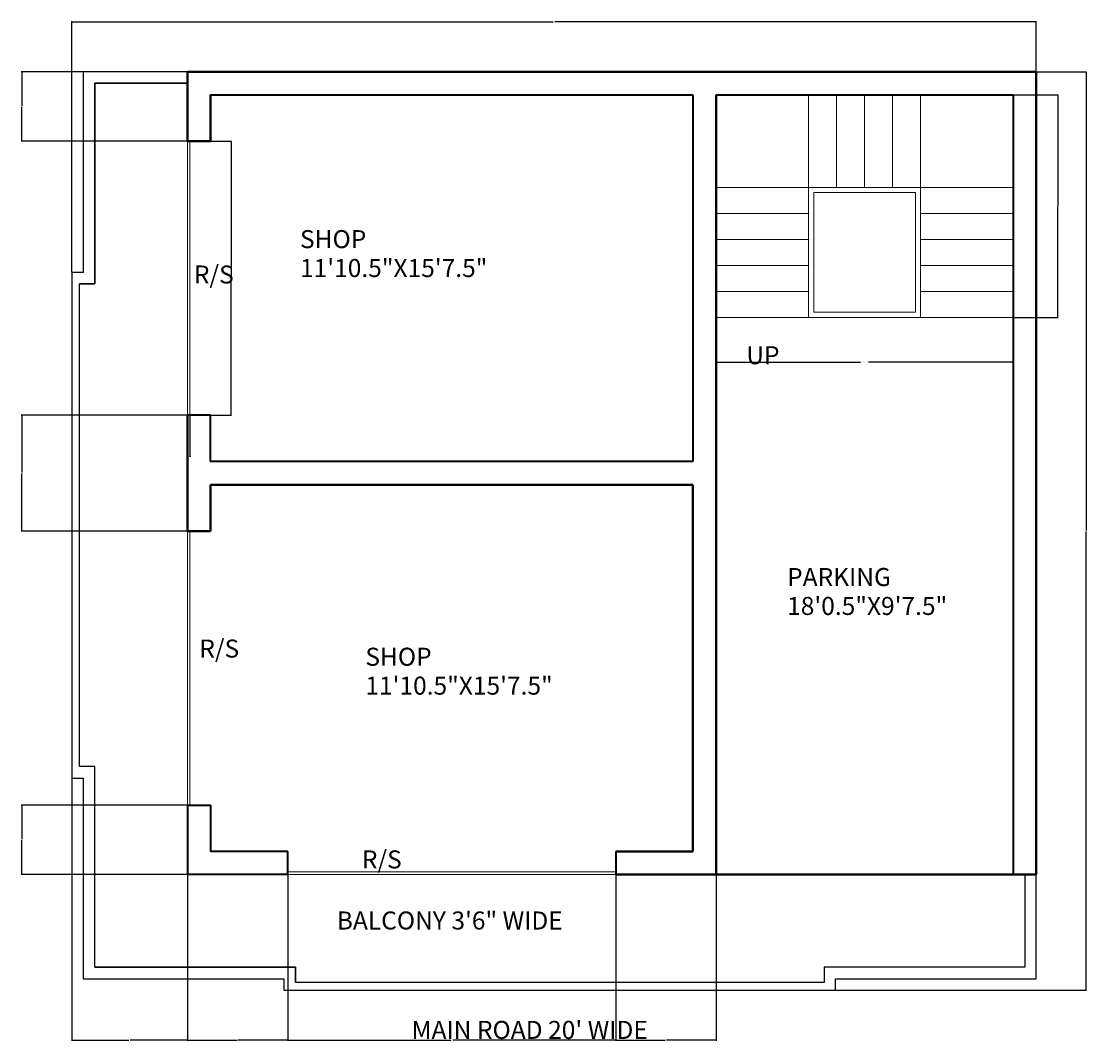
# Model space of a CAD drawing. Units: millimetres. Extents: x 2284 to 2706, y 1197 to 2041.
# Tile 3 of 3: x 2284 to 2698, y 1645 to 2041. Entities that reach past the tile are written whole.
import ezdxf

# ---------------------------------------------------------------- set-up
doc = ezdxf.new("R2010")
doc.units = ezdxf.units.MM
for name, color, linetype, lineweight in [('A-ANNO-DIMS', 2, 'Continuous', 18), ('A-ANNO-TEXT', 7, 'Continuous', 30), ('A-AREA-IDEN', 7, 'Continuous', 30), ('A-CONS', 67, 'Continuous', 13), ('A-DOOR', 7, 'Continuous', 18)]:
    doc.layers.add(name, color=color, linetype=linetype, lineweight=lineweight)
for name, color, linetype, lineweight, true_color in [('A-FLOR-STRS', 67, 'Continuous', 18, 0x727430), ('A-WALL', 11, 'Continuous', 35, 0xf27172), ('A-WALL-PRPT', 143, 'Continuous', 25, 0x7aafdf)]:
    doc.layers.add(name, color=color, linetype=linetype, lineweight=lineweight, true_color=true_color)
doc.styles.get("Standard").update_dxf_attribs({"font": 'arial.ttf'})
doc.dimstyles.get("Standard").update_dxf_attribs({"dimtxt": 0.18, "dimasz": 0.18, "dimexe": 0.18, "dimexo": 0.0625, "dimgap": 0.09, "dimtad": 0, "dimtih": 1, "dimtoh": 1, "dimdec": 4, "dimzin": 0, "dimdsep": 46, "dimtxsty": 'Standard', "dimcen": 0.09, "dimadec": 0, "dimazin": 0, "dimtfac": 1, "dimtdec": 4, "dimtofl": 0, "dimtmove": 0, "dimatfit": 3, "dimfxl": 1, "dimtolj": 1, "dimtzin": 0, "dimarcsym": 0})

# ---------------------------------------------------------------- blocks, each defined once
blk = doc.blocks.new('STAIR-U-RETURN')
for p, q in [((0, 86.5), (36, 86.5)), ((36, 86.5), (36, 50.5)), ((46.87, 50.5), (46.87, 86.5)), ((46.87, 86.5), (46.87, 50.5)), ((57.75, 50.5), (57.75, 86.5)), ((57.75, 86.5), (57.75, 50.5)), ((68.62, 50.5), (68.62, 86.5)), ((79.5, 50.5), (79.5, 86.5)), ((115.5, 50.5), (0, 50.5)), ((36, 50.5), (36, 0)), ((36, 50.5), (79.5, 50.5)), ((79.5, 0), (79.5, 50.5)), ((38, 48.5), (38, 2)), ((77.5, 48.5), (38, 48.5)), ((77.5, 2), (77.5, 48.5)), ((36, 40.4), (0, 40.4)), ((0, 40.4), (36, 40.4)), ((36, 40.4), (36, 30.3)), ((79.5, 40.4), (79.5, 30.3)), ((79.5, 40.4), (115.5, 40.4)), ((115.5, 40.4), (79.5, 40.4)), ((36, 30.3), (0, 30.3)), ((0, 30.3), (36, 30.3)), ((36, 30.3), (36, 20.2)), ((79.5, 30.3), (79.5, 20.2)), ((79.5, 30.3), (115.5, 30.3)), ((115.5, 30.3), (79.5, 30.3)), ((36, 20.2), (0, 20.2)), ((0, 20.2), (36, 20.2)), ((36, 20.2), (36, 10.1)), ((79.5, 20.2), (79.5, 10.1)), ((79.5, 20.2), (115.5, 20.2)), ((115.5, 20.2), (79.5, 20.2)), ((36, 10.1), (0, 10.1)), ((79.5, 10.1), (115.5, 10.1)), ((0, 0), (115.5, 0)), ((38, 2), (77.5, 2))]:
    blk.add_line(p, q)
blk = doc.blocks.new('DOOR-ROLL-SIDE')
for p, q in [((0, 106.5), (0, 0)), ((1, 106.5), (1, 0))]:
    blk.add_line(p, q)
blk = doc.blocks.new('*D7')
at = {"layer": 'A-ANNO-DIMS', "color": 0, "lineweight": -2, "transparency": 16777216}
for p, q in [((2554.18, 1925.73), (2554.18, 1908.29)), ((2669.68, 1925.73), (2669.68, 1908.29)), ((2554.36, 1908.47), (2610.37, 1908.47)), ((2669.5, 1908.47), (2613.49, 1908.47))]:
    blk.add_line(p, q, dxfattribs=at)
at = {"layer": 'A-ANNO-DIMS', "color": 0, "transparency": 16777216}
for points in [[(2554.36, 1908.5), (2554.36, 1908.44), (2554.18, 1908.47)], [(2669.5, 1908.5), (2669.5, 1908.44), (2669.68, 1908.47)]]:
    blk.add_solid(points, dxfattribs=at)
at = {"layer": 'Defpoints', "color": 0, "transparency": 16777216}
for p in [(2554.18, 1925.79), (2669.68, 1925.79), (2669.68, 1908.47)]:
    blk.add_point(p, dxfattribs=at)
at = {"layer": 'A-ANNO-DIMS', "color": 0, "transparency": 16777216, "insert": (2611.93, 1908.47), "char_height": 0.18, "attachment_point": 5}
blk.add_mtext('\\A1;RETURN STAIR 116 TYP.', dxfattribs=at)
blk = doc.blocks.new('*D8')
at = {"layer": 'A-ANNO-DIMS', "color": 0, "lineweight": -2, "transparency": 16777216}
for p, q in [((2669.74, 2012.29), (2687.19, 2012.29)), ((2687.01, 2012.11), (2687.01, 1969.22)), ((2687.01, 1925.97), (2687.01, 1968.86)), ((2669.74, 1925.79), (2687.19, 1925.79))]:
    blk.add_line(p, q, dxfattribs=at)
at = {"layer": 'A-ANNO-DIMS', "color": 0, "transparency": 16777216}
for points in [[(2686.98, 2012.11), (2687.04, 2012.11), (2687.01, 2012.29)], [(2686.98, 1925.97), (2687.04, 1925.97), (2687.01, 1925.79)]]:
    blk.add_solid(points, dxfattribs=at)
at = {"layer": 'Defpoints', "color": 0, "transparency": 16777216}
for p in [(2669.68, 2012.29), (2687.01, 2012.29), (2669.68, 1925.79)]:
    blk.add_point(p, dxfattribs=at)
at = {"layer": 'A-ANNO-DIMS', "color": 0, "transparency": 16777216, "insert": (2687.01, 1969.04), "char_height": 0.18, "attachment_point": 5}
blk.add_mtext('\\A1;87 TYP.', dxfattribs=at)
blk = doc.blocks.new('*D9')
at = {"layer": 'A-ANNO-DIMS', "color": 0, "lineweight": -2, "transparency": 16777216}
for p, q in [((2349.74, 1994.29), (2365.84, 1994.29)), ((2365.66, 1994.11), (2365.66, 1941.23)), ((2365.66, 1887.97), (2365.66, 1940.86)), ((2349.74, 1887.79), (2365.84, 1887.79))]:
    blk.add_line(p, q, dxfattribs=at)
at = {"layer": 'A-ANNO-DIMS', "color": 0, "transparency": 16777216}
for points in [[(2365.63, 1994.11), (2365.69, 1994.11), (2365.66, 1994.29)], [(2365.63, 1887.97), (2365.69, 1887.97), (2365.66, 1887.79)]]:
    blk.add_solid(points, dxfattribs=at)
at = {"layer": 'Defpoints', "color": 0, "transparency": 16777216}
for p in [(2349.68, 1994.29), (2365.66, 1994.29), (2349.68, 1887.79)]:
    blk.add_point(p, dxfattribs=at)
at = {"layer": 'A-ANNO-DIMS', "color": 0, "transparency": 16777216, "insert": (2365.66, 1941.04), "char_height": 0.18, "attachment_point": 5}
blk.add_mtext('\\A1;SHUTTER 107 TYP.', dxfattribs=at)
blk = doc.blocks.new('*D10')
at = {"layer": 'A-ANNO-DIMS', "color": 0, "lineweight": -2, "transparency": 16777216}
for p, q in [((2348.68, 1887.73), (2348.68, 1871.64)), ((2349.68, 1887.73), (2349.68, 1871.64)), ((2348.5, 1871.82), (2348.32, 1871.82)), ((2349.86, 1871.82), (2350.04, 1871.82))]:
    blk.add_line(p, q, dxfattribs=at)
at = {"layer": 'A-ANNO-DIMS', "color": 0, "transparency": 16777216}
for points in [[(2348.5, 1871.85), (2348.5, 1871.79), (2348.68, 1871.82)], [(2349.86, 1871.85), (2349.86, 1871.79), (2349.68, 1871.82)]]:
    blk.add_solid(points, dxfattribs=at)
at = {"layer": 'Defpoints', "color": 0, "transparency": 16777216}
for p in [(2348.68, 1887.79), (2349.68, 1887.79), (2349.68, 1871.82)]:
    blk.add_point(p, dxfattribs=at)
at = {"layer": 'A-ANNO-DIMS', "color": 0, "transparency": 16777216, "insert": (2349.18, 1871.82), "char_height": 0.18, "attachment_point": 5}
blk.add_mtext('\\A1;1 TYP.', dxfattribs=at)
blk = doc.blocks.new('*D19')
at = {"layer": 'A-ANNO-DIMS', "color": 0, "lineweight": -2, "transparency": 16777216}
for p, q in [((2303.68, 1943.35), (2303.68, 2040.87)), ((2303.86, 2040.69), (2490.89, 2040.69)), ((2678.5, 2040.69), (2491.47, 2040.69)), ((2678.68, 2021.35), (2678.68, 2040.87))]:
    blk.add_line(p, q, dxfattribs=at)
at = {"layer": 'A-ANNO-DIMS', "color": 0, "transparency": 16777216}
for points in [[(2303.86, 2040.72), (2303.86, 2040.66), (2303.68, 2040.69)], [(2678.5, 2040.72), (2678.5, 2040.66), (2678.68, 2040.69)]]:
    blk.add_solid(points, dxfattribs=at)
at = {"layer": 'Defpoints', "color": 0, "transparency": 16777216}
for p in [(2678.68, 2040.69), (2678.68, 2021.29), (2303.68, 1943.29)]:
    blk.add_point(p, dxfattribs=at)
at = {"layer": 'A-ANNO-DIMS', "color": 0, "transparency": 16777216, "insert": (2491.18, 2040.69), "char_height": 0.18, "attachment_point": 5}
blk.add_mtext('\\A1;375', dxfattribs=at)
blk = doc.blocks.new('*D20')
at = {"layer": 'A-ANNO-DIMS', "color": 0, "lineweight": -2, "transparency": 16777216}
for p, q in [((2678.74, 2021.29), (2698.26, 2021.29)), ((2698.08, 2021.11), (2698.08, 1842.97)), ((2698.08, 1664.47), (2698.08, 1842.61)), ((2600.74, 1664.29), (2698.26, 1664.29))]:
    blk.add_line(p, q, dxfattribs=at)
at = {"layer": 'A-ANNO-DIMS', "color": 0, "transparency": 16777216}
for points in [[(2698.05, 2021.11), (2698.11, 2021.11), (2698.08, 2021.29)], [(2698.05, 1664.47), (2698.11, 1664.47), (2698.08, 1664.29)]]:
    blk.add_solid(points, dxfattribs=at)
at = {"layer": 'Defpoints', "color": 0, "transparency": 16777216}
for p in [(2678.68, 2021.29), (2698.08, 2021.29), (2600.68, 1664.29)]:
    blk.add_point(p, dxfattribs=at)
at = {"layer": 'A-ANNO-DIMS', "color": 0, "transparency": 16777216, "insert": (2698.08, 1842.79), "char_height": 0.18, "attachment_point": 5}
blk.add_mtext('\\A1;357', dxfattribs=at)
blk = doc.blocks.new('*D21')
at = {"layer": 'A-ANNO-DIMS', "color": 0, "lineweight": -2, "transparency": 16777216}
for p, q in [((2348.62, 2021.29), (2284.1, 2021.29)), ((2284.28, 2021.11), (2284.28, 2007.97)), ((2284.28, 1994.47), (2284.28, 2007.61)), ((2348.62, 1994.29), (2284.1, 1994.29))]:
    blk.add_line(p, q, dxfattribs=at)
at = {"layer": 'A-ANNO-DIMS', "color": 0, "transparency": 16777216}
for points in [[(2284.25, 2021.11), (2284.31, 2021.11), (2284.28, 2021.29)], [(2284.25, 1994.47), (2284.31, 1994.47), (2284.28, 1994.29)]]:
    blk.add_solid(points, dxfattribs=at)
at = {"layer": 'Defpoints', "color": 0, "transparency": 16777216}
for p in [(2284.28, 2021.29), (2348.68, 2021.29), (2348.68, 1994.29)]:
    blk.add_point(p, dxfattribs=at)
at = {"layer": 'A-ANNO-DIMS', "color": 0, "transparency": 16777216, "insert": (2284.28, 2007.79), "char_height": 0.18, "attachment_point": 5}
blk.add_mtext('\\A1;27', dxfattribs=at)
blk = doc.blocks.new('*D22')
at = {"layer": 'A-ANNO-DIMS', "color": 0, "lineweight": -2, "transparency": 16777216}
for p, q in [((2348.62, 1887.79), (2284.1, 1887.79)), ((2284.28, 1887.61), (2284.28, 1865.47)), ((2284.28, 1842.97), (2284.28, 1865.11)), ((2348.62, 1842.79), (2284.1, 1842.79))]:
    blk.add_line(p, q, dxfattribs=at)
at = {"layer": 'A-ANNO-DIMS', "color": 0, "transparency": 16777216}
for points in [[(2284.25, 1887.61), (2284.31, 1887.61), (2284.28, 1887.79)], [(2284.25, 1842.97), (2284.31, 1842.97), (2284.28, 1842.79)]]:
    blk.add_solid(points, dxfattribs=at)
at = {"layer": 'Defpoints', "color": 0, "transparency": 16777216}
for p in [(2284.28, 1887.79), (2348.68, 1887.79), (2348.68, 1842.79)]:
    blk.add_point(p, dxfattribs=at)
at = {"layer": 'A-ANNO-DIMS', "color": 0, "transparency": 16777216, "insert": (2284.28, 1865.29), "char_height": 0.18, "attachment_point": 5}
blk.add_mtext('\\A1;45', dxfattribs=at)
blk = doc.blocks.new('*D23')
at = {"layer": 'A-ANNO-DIMS', "color": 0, "lineweight": -2, "transparency": 16777216}
for p, q in [((2348.62, 1736.29), (2284.1, 1736.29)), ((2284.28, 1736.11), (2284.28, 1722.97)), ((2284.28, 1709.47), (2284.28, 1722.61)), ((2348.62, 1709.29), (2284.1, 1709.29))]:
    blk.add_line(p, q, dxfattribs=at)
at = {"layer": 'A-ANNO-DIMS', "color": 0, "transparency": 16777216}
for points in [[(2284.25, 1736.11), (2284.31, 1736.11), (2284.28, 1736.29)], [(2284.25, 1709.47), (2284.31, 1709.47), (2284.28, 1709.29)]]:
    blk.add_solid(points, dxfattribs=at)
at = {"layer": 'Defpoints', "color": 0, "transparency": 16777216}
for p in [(2284.28, 1736.29), (2348.68, 1736.29), (2348.68, 1709.29)]:
    blk.add_point(p, dxfattribs=at)
at = {"layer": 'A-ANNO-DIMS', "color": 0, "transparency": 16777216, "insert": (2284.28, 1722.79), "char_height": 0.18, "attachment_point": 5}
blk.add_mtext('\\A1;27', dxfattribs=at)
blk = doc.blocks.new('*D24')
at = {"layer": 'A-ANNO-DIMS', "color": 0, "lineweight": -2, "transparency": 16777216}
for p, q in [((2303.68, 1746.73), (2303.68, 1644.71)), ((2348.68, 1709.23), (2348.68, 1644.71)), ((2303.86, 1644.89), (2325.96, 1644.89)), ((2348.5, 1644.89), (2326.4, 1644.89))]:
    blk.add_line(p, q, dxfattribs=at)
at = {"layer": 'A-ANNO-DIMS', "color": 0, "transparency": 16777216}
for points in [[(2303.86, 1644.92), (2303.86, 1644.86), (2303.68, 1644.89)], [(2348.5, 1644.92), (2348.5, 1644.86), (2348.68, 1644.89)]]:
    blk.add_solid(points, dxfattribs=at)
at = {"layer": 'Defpoints', "color": 0, "transparency": 16777216}
for p in [(2303.68, 1746.79), (2348.68, 1709.29), (2348.68, 1644.89)]:
    blk.add_point(p, dxfattribs=at)
at = {"layer": 'A-ANNO-DIMS', "color": 0, "transparency": 16777216, "insert": (2326.18, 1644.89), "char_height": 0.18, "attachment_point": 5}
blk.add_mtext('\\A1;45', dxfattribs=at)
blk = doc.blocks.new('*D25')
at = {"layer": 'A-ANNO-DIMS', "color": 0, "lineweight": -2, "transparency": 16777216}
for p, q in [((2348.68, 1709.23), (2348.68, 1644.71)), ((2387.68, 1709.23), (2387.68, 1644.71)), ((2348.86, 1644.89), (2367.96, 1644.89)), ((2387.5, 1644.89), (2368.4, 1644.89))]:
    blk.add_line(p, q, dxfattribs=at)
at = {"layer": 'A-ANNO-DIMS', "color": 0, "transparency": 16777216}
for points in [[(2348.86, 1644.92), (2348.86, 1644.86), (2348.68, 1644.89)], [(2387.5, 1644.92), (2387.5, 1644.86), (2387.68, 1644.89)]]:
    blk.add_solid(points, dxfattribs=at)
at = {"layer": 'Defpoints', "color": 0, "transparency": 16777216}
for p in [(2348.68, 1709.29), (2387.68, 1709.29), (2387.68, 1644.89)]:
    blk.add_point(p, dxfattribs=at)
at = {"layer": 'A-ANNO-DIMS', "color": 0, "transparency": 16777216, "insert": (2368.18, 1644.89), "char_height": 0.18, "attachment_point": 5}
blk.add_mtext('\\A1;39', dxfattribs=at)
blk = doc.blocks.new('*D26')
at = {"layer": 'A-ANNO-DIMS', "color": 0, "lineweight": -2, "transparency": 16777216}
for p, q in [((2387.68, 1709.23), (2387.68, 1644.71)), ((2515.18, 1709.23), (2515.18, 1644.71)), ((2387.86, 1644.89), (2451.04, 1644.89)), ((2515, 1644.89), (2451.82, 1644.89))]:
    blk.add_line(p, q, dxfattribs=at)
at = {"layer": 'A-ANNO-DIMS', "color": 0, "transparency": 16777216}
for points in [[(2387.86, 1644.92), (2387.86, 1644.86), (2387.68, 1644.89)], [(2515, 1644.92), (2515, 1644.86), (2515.18, 1644.89)]]:
    blk.add_solid(points, dxfattribs=at)
at = {"layer": 'Defpoints', "color": 0, "transparency": 16777216}
for p in [(2387.68, 1709.29), (2515.18, 1709.29), (2515.18, 1644.89)]:
    blk.add_point(p, dxfattribs=at)
at = {"layer": 'A-ANNO-DIMS', "color": 0, "transparency": 16777216, "insert": (2451.43, 1644.89), "char_height": 0.18, "attachment_point": 5}
blk.add_mtext('\\A1;127.5', dxfattribs=at)
blk = doc.blocks.new('*D27')
at = {"layer": 'A-ANNO-DIMS', "color": 0, "lineweight": -2, "transparency": 16777216}
for p, q in [((2515.18, 1709.23), (2515.18, 1644.71)), ((2554.18, 1709.23), (2554.18, 1644.71)), ((2515.36, 1644.89), (2534.46, 1644.89)), ((2554, 1644.89), (2534.9, 1644.89))]:
    blk.add_line(p, q, dxfattribs=at)
at = {"layer": 'A-ANNO-DIMS', "color": 0, "transparency": 16777216}
for points in [[(2515.36, 1644.92), (2515.36, 1644.86), (2515.18, 1644.89)], [(2554, 1644.92), (2554, 1644.86), (2554.18, 1644.89)]]:
    blk.add_solid(points, dxfattribs=at)
at = {"layer": 'Defpoints', "color": 0, "transparency": 16777216}
for p in [(2515.18, 1709.29), (2554.18, 1709.29), (2554.18, 1644.89)]:
    blk.add_point(p, dxfattribs=at)
at = {"layer": 'A-ANNO-DIMS', "color": 0, "transparency": 16777216, "insert": (2534.68, 1644.89), "char_height": 0.18, "attachment_point": 5}
blk.add_mtext('\\A1;39', dxfattribs=at)

msp = doc.modelspace()

# ---------------------------------------------------------------- linework, layer by layer
at = {"layer": 'A-CONS'}
for p in [(2601.06, 1976.29), (2611.93, 1976.29), (2622.81, 1976.29), (2590.18, 1966.19), (2633.68, 1966.19), (2590.18, 1956.09), (2633.68, 1956.09), (2590.18, 1945.99), (2633.68, 1945.99), (2590.18, 1935.89), (2633.68, 1935.89)]:
    msp.add_point(p, dxfattribs=at)
at = {"layer": 'A-DOOR'}
for p, q in [((2349.68, 1736.29), (2348.68, 1736.29)), ((2349.68, 1736.29), (2348.68, 1736.29)), ((2349.68, 1736.29), (2348.68, 1736.29)), ((2387.68, 1710.29), (2387.68, 1709.29)), ((2387.68, 1710.29), (2515.18, 1710.29)), ((2387.68, 1709.29), (2515.18, 1709.29))]:
    msp.add_line(p, q, dxfattribs=at)
at = {"layer": 'A-FLOR-STRS'}
for p, q in [((2554.18, 2012.29), (2584.18, 2012.29)), ((2554.18, 2012.29), (2554.18, 1982.29)), ((2590.18, 2012.29), (2590.18, 1976.29)), ((2669.68, 2012.29), (2633.68, 2012.29)), ((2633.68, 2012.29), (2633.68, 1976.29)), ((2669.68, 2012.29), (2639.68, 2012.29)), ((2601.06, 1976.29), (2611.93, 1976.29)), ((2611.93, 1976.29), (2622.81, 1976.29)), ((2631.68, 1976.29), (2669.68, 1976.29)), ((2633.68, 1976.29), (2633.68, 1925.79)), ((2592.18, 1927.79), (2592.18, 1974.29)), ((2592.18, 1974.29), (2631.68, 1974.29)), ((2631.68, 1974.29), (2631.68, 1927.79)), ((2592.18, 1927.79), (2631.68, 1927.79)), ((2590.18, 1925.79), (2554.18, 1925.79)), ((2590.18, 1925.79), (2633.68, 1925.79)), ((2590.18, 1925.79), (2633.68, 1925.79)), ((2669.68, 1925.79), (2633.68, 1925.79))]:
    msp.add_line(p, q, dxfattribs=at)
at = {"layer": 'A-WALL'}
for p, q in [((2348.68, 2021.29), (2678.68, 2021.29)), ((2348.68, 2021.29), (2357.68, 2021.29)), ((2348.68, 1994.29), (2348.68, 2021.29)), ((2678.68, 2021.29), (2348.68, 2021.29)), ((2348.68, 2021.29), (2348.68, 1994.29)), ((2678.68, 2021.29), (2678.68, 1709.29)), ((2678.68, 1709.29), (2678.68, 2021.29)), ((2357.68, 2012.29), (2545.18, 2012.29)), ((2357.68, 2012.29), (2545.18, 2012.29)), ((2357.68, 2012.29), (2357.68, 1994.29)), ((2357.68, 1994.29), (2357.68, 2012.29)), ((2357.68, 1994.29), (2357.68, 2012.29)), ((2357.68, 2012.29), (2545.18, 2012.29)), ((2545.18, 2012.29), (2545.18, 1869.79)), ((2545.18, 2012.29), (2545.18, 1869.79)), ((2554.18, 2012.29), (2669.68, 2012.29)), ((2554.18, 1925.79), (2554.18, 2012.29)), ((2554.18, 2012.29), (2554.18, 1925.79)), ((2554.18, 1709.29), (2554.18, 2012.29)), ((2554.18, 2012.29), (2669.68, 2012.29)), ((2669.68, 2012.29), (2669.68, 1925.79)), ((2669.68, 2012.29), (2669.68, 1709.29)), ((2357.68, 1994.29), (2348.68, 1994.29)), ((2348.68, 1994.29), (2357.68, 1994.29)), ((2554.18, 1925.79), (2554.18, 1709.29)), ((2669.68, 1925.79), (2669.68, 1709.29)), ((2357.68, 1887.79), (2348.68, 1887.79)), ((2348.68, 1842.79), (2348.68, 1887.79)), ((2357.68, 1887.79), (2348.68, 1887.79)), ((2348.68, 1887.79), (2348.68, 1842.79)), ((2357.68, 1869.79), (2357.68, 1887.79)), ((2357.68, 1869.79), (2357.68, 1887.79)), ((2357.68, 1878.79), (2357.68, 1887.79)), ((2357.68, 1869.79), (2357.68, 1878.79)), ((2545.18, 1869.79), (2357.68, 1869.79)), ((2545.18, 1869.79), (2357.68, 1869.79)), ((2545.18, 1860.79), (2357.68, 1860.79)), ((2357.68, 1860.79), (2357.68, 1842.79)), ((2357.68, 1860.79), (2357.68, 1842.79)), ((2357.68, 1842.79), (2357.68, 1860.79)), ((2357.68, 1860.79), (2545.18, 1860.79)), ((2545.18, 1718.29), (2545.18, 1860.79)), ((2545.18, 1860.79), (2545.18, 1718.29)), ((2357.68, 1842.79), (2348.68, 1842.79)), ((2348.68, 1842.79), (2357.68, 1842.79)), ((2348.68, 1736.29), (2348.68, 1709.29)), ((2348.68, 1736.29), (2357.68, 1736.29)), ((2357.68, 1736.29), (2357.68, 1718.29)), ((2387.68, 1718.29), (2357.68, 1718.29)), ((2387.68, 1709.29), (2387.68, 1718.29)), ((2545.18, 1718.29), (2515.18, 1718.29)), ((2515.18, 1718.29), (2515.18, 1709.29)), ((2515.18, 1718.29), (2545.18, 1718.29)), ((2545.18, 1718.29), (2515.18, 1718.29)), ((2515.18, 1718.29), (2515.18, 1709.29)), ((2387.68, 1709.29), (2348.68, 1709.29)), ((2678.68, 1709.29), (2515.18, 1709.29)), ((2515.18, 1709.29), (2554.18, 1709.29)), ((2554.18, 1709.29), (2545.18, 1709.29)), ((2669.68, 1709.29), (2554.18, 1709.29)), ((2554.18, 1709.29), (2678.68, 1709.29))]:
    msp.add_line(p, q, dxfattribs=at)
at = {"layer": 'A-WALL-PRPT'}
for p, q in [((2348.68, 2021.29), (2308.18, 2021.29)), ((2308.18, 2021.29), (2308.18, 1943.29)), ((2348.68, 2021.29), (2308.18, 2021.29)), ((2308.18, 2021.29), (2308.18, 1943.29)), ((2348.68, 2016.79), (2312.68, 2016.79)), ((2312.68, 2016.79), (2312.68, 1938.79)), ((2312.68, 1938.79), (2312.68, 2016.79)), ((2312.68, 2016.79), (2348.68, 2016.79)), ((2308.18, 1943.29), (2303.68, 1943.29)), ((2303.68, 1943.29), (2303.68, 1751.29)), ((2308.18, 1943.29), (2303.68, 1943.29)), ((2303.68, 1943.29), (2303.68, 1746.79)), ((2312.68, 1938.79), (2306.68, 1938.79)), ((2306.68, 1751.29), (2306.68, 1938.79)), ((2306.68, 1751.29), (2306.68, 1938.79)), ((2306.68, 1938.79), (2312.68, 1938.79)), ((2303.68, 1751.29), (2303.68, 1746.79)), ((2312.68, 1751.29), (2306.68, 1751.29)), ((2308.18, 1751.29), (2306.68, 1751.29)), ((2312.68, 1751.29), (2308.18, 1751.29)), ((2312.68, 1673.29), (2312.68, 1751.29)), ((2312.68, 1673.29), (2312.68, 1751.29)), ((2303.68, 1746.79), (2308.18, 1746.79)), ((2303.68, 1746.79), (2308.18, 1746.79)), ((2308.18, 1746.79), (2308.18, 1673.29)), ((2308.18, 1746.79), (2308.18, 1668.79)), ((2674.18, 1709.29), (2674.18, 1673.29)), ((2674.18, 1709.29), (2674.18, 1673.29)), ((2678.68, 1668.79), (2678.68, 1709.29)), ((2678.68, 1668.79), (2678.68, 1709.29)), ((2308.18, 1673.29), (2308.18, 1668.79)), ((2348.68, 1673.29), (2312.68, 1673.29)), ((2312.68, 1673.29), (2390.68, 1673.29)), ((2390.68, 1673.29), (2312.68, 1673.29)), ((2390.68, 1673.29), (2390.68, 1667.29)), ((2390.68, 1667.29), (2390.68, 1673.29)), ((2674.18, 1673.29), (2596.18, 1673.29)), ((2596.18, 1673.29), (2596.18, 1667.29)), ((2674.18, 1673.29), (2596.18, 1673.29)), ((2596.18, 1673.29), (2596.18, 1667.29)), ((2308.18, 1668.79), (2386.18, 1668.79)), ((2308.18, 1668.79), (2386.18, 1668.79)), ((2386.18, 1668.79), (2386.18, 1664.29)), ((2386.18, 1668.79), (2386.18, 1664.29)), ((2596.18, 1667.29), (2390.68, 1667.29)), ((2596.18, 1667.29), (2390.68, 1667.29)), ((2600.68, 1664.29), (2600.68, 1668.79)), ((2600.68, 1668.79), (2674.18, 1668.79)), ((2600.68, 1664.29), (2600.68, 1668.79)), ((2600.68, 1668.79), (2678.68, 1668.79)), ((2674.18, 1668.79), (2678.68, 1668.79)), ((2386.18, 1664.29), (2596.18, 1664.29)), ((2386.18, 1664.29), (2598.43, 1664.29)), ((2596.18, 1664.29), (2600.68, 1664.29)), ((2598.43, 1664.29), (2600.68, 1664.29))]:
    msp.add_line(p, q, dxfattribs=at)

# ---------------------------------------------------------------- block references
at = {"layer": 'A-DOOR'}
for p in [(2348.68, 1887.79), (2348.68, 1736.29)]:
    msp.add_blockref('DOOR-ROLL-SIDE', p, dxfattribs=at)
at = {"layer": 'A-FLOR-STRS'}
msp.add_blockref('STAIR-U-RETURN', (2554.18, 1925.79), dxfattribs=at)

# ---------------------------------------------------------------- texts
at = {"layer": 'A-ANNO-TEXT'}
for s, p in [('R/S', (2351.18, 1938.98)), ('UP', (2565.94, 1907.6)), ('R/S', (2353.3, 1793.6)), ('R/S', (2416.49, 1711.66)), ("MAIN ROAD 20' WIDE", (2435.83, 1645.4))]:
    msp.add_text(s, height=7, dxfattribs=at).set_placement(p)
at = {"layer": 'A-AREA-IDEN'}
for s, p in [('SHOP', (2392.45, 1952.73)), ('11\'10.5"X15\'7.5"', (2392.45, 1941.49)), ('PARKING', (2581.82, 1821.41)), ('18\'0.5"X9\'7.5"', (2581.82, 1810.16)), ('SHOP', (2417.85, 1790.43)), ('11\'10.5"X15\'7.5"', (2417.85, 1779.19)), ('BALCONY 3\'6" WIDE', (2406.74, 1687.92))]:
    msp.add_text(s, height=7, dxfattribs=at).set_placement(p)

# ---------------------------------------------------------------- dimensions: what is measured, and where the dimension line sits
at = {"layer": 'A-ANNO-DIMS'}
for base, p1, p2, override, picture, middle in [((2678.68, 2040.69), (2303.68, 1943.29), (2678.68, 2021.29), {"dimdec": 0, "dimlfac": 1, "dimrnd": 0, "dimzin": 0, "dimdsep": 46, "dimlunit": 2}, '*D19', (2491.18, 2040.69)), ((2348.68, 1644.89), (2303.68, 1746.79), (2348.68, 1709.29), {"dimdec": 0, "dimlfac": 1, "dimrnd": 0, "dimzin": 0, "dimdsep": 46, "dimlunit": 2}, '*D24', (2326.18, 1644.89)), ((2387.68, 1644.89), (2348.68, 1709.29), (2387.68, 1709.29), {"dimdec": 0, "dimlfac": 1, "dimrnd": 0, "dimzin": 0, "dimdsep": 46, "dimlunit": 2}, '*D25', (2368.18, 1644.89)), ((2515.18, 1644.89), (2387.68, 1709.29), (2515.18, 1709.29), {"dimdec": 1, "dimlfac": 1, "dimrnd": 0, "dimzin": 0, "dimdsep": 46, "dimlunit": 2}, '*D26', (2451.43, 1644.89)), ((2554.18, 1644.89), (2515.18, 1709.29), (2554.18, 1709.29), {"dimdec": 0, "dimlfac": 1, "dimrnd": 0, "dimzin": 0, "dimdsep": 46, "dimlunit": 2}, '*D27', (2534.68, 1644.89))]:
    dim = msp.add_linear_dim(base=base, p1=p1, p2=p2, dimstyle='Standard', override=override, dxfattribs=at)
    dim.commit()
    dim.dimension.update_dxf_attribs({"geometry": picture, "text_midpoint": middle})
for base, p1, p2, picture, middle in [((2284.28, 2021.29), (2348.68, 1994.29), (2348.68, 2021.29), '*D21', (2284.28, 2007.79)), ((2698.08, 2021.29), (2600.68, 1664.29), (2678.68, 2021.29), '*D20', (2698.08, 1842.79)), ((2284.28, 1887.79), (2348.68, 1842.79), (2348.68, 1887.79), '*D22', (2284.28, 1865.29)), ((2284.28, 1736.29), (2348.68, 1709.29), (2348.68, 1736.29), '*D23', (2284.28, 1722.79))]:
    dim = msp.add_linear_dim(base=base, p1=p1, p2=p2, angle=90, dimstyle='Standard', override={"dimdec": 0, "dimlfac": 1, "dimrnd": 0, "dimzin": 0, "dimdsep": 46, "dimlunit": 2}, dxfattribs=at)
    dim.commit()
    dim.dimension.update_dxf_attribs({"geometry": picture, "text_midpoint": middle})
for base, p1, p2, text, picture, middle in [((2687.0055728, 2012.29209695), (2669.6805728, 1925.79209695), (2669.6805728, 2012.29209695), '<> TYP.', '*D8', (2687.0055728, 1969.04209695)), ((2365.6555728, 1994.29209695), (2349.6805728, 1887.79209695), (2349.6805728, 1994.29209695), 'SHUTTER <> TYP.', '*D9', (2365.6555728, 1941.04209695))]:
    dim = msp.add_linear_dim(base=base, p1=p1, p2=p2, angle=90, text=text, dimstyle='Standard', override={"dimdec": 0, "dimlfac": 1, "dimrnd": 0, "dimzin": 0, "dimdsep": 46, "dimlunit": 2}, dxfattribs=at)
    dim.commit()
    dim.dimension.update_dxf_attribs({"geometry": picture, "text_midpoint": middle})
for base, p1, p2, text, picture, middle in [((2669.6805728, 1908.46709695), (2554.1805728, 1925.79209695), (2669.6805728, 1925.79209695), 'RETURN STAIR <> TYP.', '*D7', (2611.9305728, 1908.46709695)), ((2349.68, 1871.82), (2348.68, 1887.79), (2349.68, 1887.79), '<> TYP.', '*D10', (2349.18, 1871.82))]:
    dim = msp.add_linear_dim(base=base, p1=p1, p2=p2, text=text, dimstyle='Standard', override={"dimdec": 0, "dimlfac": 1, "dimrnd": 0, "dimzin": 0, "dimdsep": 46, "dimlunit": 2}, dxfattribs=at)
    dim.commit()
    dim.dimension.update_dxf_attribs({"geometry": picture, "text_midpoint": middle})

doc.saveas('drawing.dxf')
